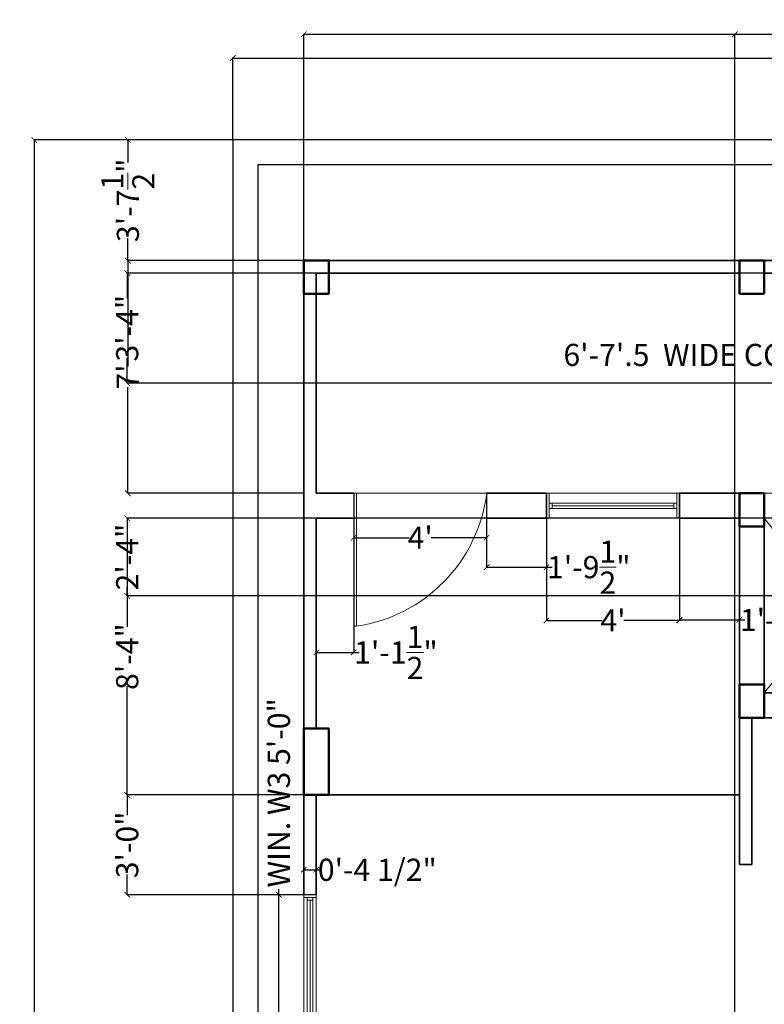
# Model space of a CAD drawing. Units: inches. Extents: x 490 to 1091, y 501 to 1322.
# Tile 4 of 5: x 490 to 759, y 959 to 1314. Entities that reach past the tile are written whole.
import ezdxf

# ---------------------------------------------------------------- set-up
doc = ezdxf.new("R2010")
doc.units = ezdxf.units.IN
doc.header["$MEASUREMENT"] = 0
doc.linetypes.add('ACAD_ISO02W100', pattern=[15, 12, -3])
for name, color, linetype, lineweight in [('A-ANNO-DIMS', 2, 'Continuous', 18), ('A-AREA-IDEN', 7, 'Continuous', 25), ('A-COLS', 12, 'Continuous', 50), ('A-DOOR', 3, 'Continuous', 20), ('A-EQPM-EVTR', 152, 'Continuous', 20), ('A-EQPM-EVTR-HIDN', 152, 'ACAD_ISO02W100', 13), ('A-GLAZ', 4, 'Continuous', 18), ('A-WALL', 7, 'Continuous', 35), ('C-PROP', 8, 'Continuous', 25)]:
    doc.layers.add(name, color=color, linetype=linetype, lineweight=lineweight)
doc.styles.get("Standard").update_dxf_attribs({"font": 'arial.ttf'})
doc.dimstyles.get("Standard").update_dxf_attribs({"dimtxt": 8, "dimasz": 2, "dimexe": 0.18, "dimexo": 0.0625, "dimgap": 0.09, "dimtad": 0, "dimdec": 1, "dimzin": 0, "dimdsep": 46, "dimlunit": 4, "dimtxsty": 'Standard', "dimblk": 'ARCHTICK', "dimcen": 0.09, "dimadec": 0, "dimazin": 0, "dimtfac": 1, "dimtdec": 1, "dimtofl": 0, "dimtmove": 0, "dimatfit": 3, "dimldrblk": 'ARCHTICK', "dimfxl": 1, "dimtolj": 1, "dimtzin": 0, "dimarcsym": 0})

# ---------------------------------------------------------------- blocks, each defined once
blk = doc.blocks.new('_ArchTick')
at = {"color": 0, "linetype": 'ByBlock', "const_width": 0.15}
blk.add_lwpolyline([(-0.5, -0.5), (0.5, 0.5)], dxfattribs=at)
blk = doc.blocks.new('*D2')
at = {"layer": 'A-ANNO-DIMS', "color": 0, "lineweight": -2, "transparency": 16777216}
for p, q in [((592.81, 1227.28), (529.2, 1227.28)), ((529.38, 1227.28), (529.38, 1189.02)), ((529.38, 1143.28), (529.38, 1181.55)), ((592.81, 1143.28), (529.2, 1143.28))]:
    blk.add_line(p, q, dxfattribs=at)
at = {"layer": 'Defpoints', "color": 0, "transparency": 16777216}
for p in [(592.87, 1227.28), (529.38, 1143.28), (592.87, 1143.28)]:
    blk.add_point(p, dxfattribs=at)
at = {"layer": 'A-ANNO-DIMS', "color": 0, "lineweight": -2, "transparency": 16777216, "xscale": 2, "yscale": 2, "zscale": 2}
for p, rotation in [((529.38, 1227.28), 90), ((529.38, 1143.28), 270)]:
    blk.add_blockref('_ArchTick', p, dxfattribs=dict(at, rotation=rotation))
at = {"layer": 'A-ANNO-DIMS', "color": 0, "transparency": 16777216, "insert": (529.38, 1185.28), "char_height": 8, "attachment_point": 5, "rotation": 90}
blk.add_mtext("\\A1;7'", dxfattribs=at)
blk = doc.blocks.new('*D3')
at = {"layer": 'A-ANNO-DIMS', "color": 0, "lineweight": -2, "transparency": 16777216}
for p, q in [((567.27, 1270.95), (567.27, 1300.61)), ((567.27, 1300.43), (800.23, 1300.43)), ((1047.27, 1300.43), (814.31, 1300.43)), ((1047.27, 1270.95), (1047.27, 1300.61))]:
    blk.add_line(p, q, dxfattribs=at)
at = {"layer": 'Defpoints', "color": 0, "transparency": 16777216}
for p in [(567.27, 1300.43), (567.27, 1270.88), (1047.27, 1270.88)]:
    blk.add_point(p, dxfattribs=at)
at = {"layer": 'A-ANNO-DIMS', "color": 0, "lineweight": -2, "transparency": 16777216, "xscale": 2, "yscale": 2, "zscale": 2, "rotation": 180}
blk.add_blockref('_ArchTick', (567.27, 1300.43), dxfattribs=at)
at = {"layer": 'A-ANNO-DIMS', "color": 0, "lineweight": -2, "transparency": 16777216, "xscale": 2, "yscale": 2, "zscale": 2}
blk.add_blockref('_ArchTick', (1047.27, 1300.43), dxfattribs=at)
at = {"layer": 'A-ANNO-DIMS', "color": 0, "transparency": 16777216, "insert": (807.27, 1300.43), "char_height": 8, "attachment_point": 5}
blk.add_mtext("\\A1;40'", dxfattribs=at)
blk = doc.blocks.new('*D4')
at = {"layer": 'A-ANNO-DIMS', "color": 0, "lineweight": -2, "transparency": 16777216}
for p, q in [((567.21, 1270.88), (495.41, 1270.88)), ((495.59, 1270.88), (495.59, 917.79)), ((495.59, 550.88), (495.59, 903.98)), ((567.21, 550.88), (495.41, 550.88))]:
    blk.add_line(p, q, dxfattribs=at)
at = {"layer": 'Defpoints', "color": 0, "transparency": 16777216}
for p in [(567.27, 1270.88), (495.59, 550.88), (567.27, 550.88)]:
    blk.add_point(p, dxfattribs=at)
at = {"layer": 'A-ANNO-DIMS', "color": 0, "lineweight": -2, "transparency": 16777216, "xscale": 2, "yscale": 2, "zscale": 2}
for p, rotation in [((495.59, 1270.88), 90), ((495.59, 550.88), 270)]:
    blk.add_blockref('_ArchTick', p, dxfattribs=dict(at, rotation=rotation))
at = {"layer": 'A-ANNO-DIMS', "color": 0, "transparency": 16777216, "insert": (495.59, 910.88), "char_height": 8, "attachment_point": 5, "rotation": 90}
blk.add_mtext("\\A1;60'", dxfattribs=at)
blk = doc.blocks.new('bnfgfhvhm')
for p, q in [((1106.43, 1203.63), (1115.43, 1203.63)), ((1106.43, 1191.63), (1106.43, 1203.63)), ((1115.43, 1203.63), (1115.43, 1191.63)), ((1115.43, 1191.63), (1106.43, 1191.63))]:
    blk.add_line(p, q)
blk = doc.blocks.new('ghthyjutyut')
for p, q in [((1385.5, 1212.32), (1433.5, 1212.32)), ((1385.5, 1203.32), (1385.5, 1212.32)), ((1386.5, 1203.32), (1386.5, 1212.32)), ((1432.5, 1212.32), (1432.5, 1203.32)), ((1433.5, 1212.32), (1433.5, 1203.32)), ((1386.5, 1208.82), (1432.5, 1208.82)), ((1387.5, 1206.82), (1387.5, 1208.82)), ((1431.5, 1208.82), (1431.5, 1206.82)), ((1386.5, 1206.82), (1432.5, 1206.82)), ((1387.5, 1207.82), (1431.5, 1207.82)), ((1433.5, 1203.32), (1385.5, 1203.32))]:
    blk.add_line(p, q)
blk = doc.blocks.new('jcjg  bmvh')
for p, q in [((1232.66, 1066.6), (1223.66, 1066.6)), ((1223.66, 1066.6), (1223.66, 1042.6)), ((1232.66, 1042.6), (1232.66, 1066.6)), ((1223.66, 1042.6), (1232.66, 1042.6))]:
    blk.add_line(p, q)
blk = doc.blocks.new('ggnhgjgfjhgjjjjjjjj')
for p, q in [((597.37, 998.37), (592.87, 998.37)), ((592.87, 998.37), (592.87, 938.37)), ((597.37, 998.37), (592.87, 998.37)), ((597.37, 997.37), (592.87, 997.37)), ((594.12, 997.37), (594.12, 939.37)), ((596.12, 996.37), (594.12, 996.37)), ((595.12, 996.37), (595.12, 940.37)), ((596.12, 997.37), (596.12, 939.37)), ((597.37, 938.37), (597.37, 998.37)), ((592.87, 939.37), (597.37, 939.37)), ((594.12, 940.37), (596.12, 940.37)), ((597.37, 938.37), (592.87, 938.37)), ((592.87, 938.37), (597.37, 938.37))]:
    blk.add_line(p, q)
blk = doc.blocks.new("door4'")
for p, q in [((1439.4, 1060.56), (1439.4, 1108.56)), ((1439.4, 1108.56), (1440.4, 1108.56)), ((1440.4, 1108.56), (1440.4, 1060.56)), ((1439.4, 1060.56), (1487.4, 1060.56))]:
    blk.add_line(p, q)
blk.add_arc((1432.28, 1053.6), 55.56, 7.2031, 81.5907)
blk = doc.blocks.new('*D26')
at = {"layer": 'A-ANNO-DIMS', "color": 0, "lineweight": -2, "transparency": 16777216}
for p, q in [((728.47, 1134.22), (728.47, 1097.37)), ((750.07, 1134.22), (750.07, 1097.37)), ((728.47, 1097.55), (750.07, 1097.55)), ((750.07, 1097.55), (752.07, 1097.55))]:
    blk.add_line(p, q, dxfattribs=at)
at = {"layer": 'Defpoints', "color": 0, "transparency": 16777216}
for p in [(728.47, 1134.28), (750.07, 1134.28), (750.07, 1097.55)]:
    blk.add_point(p, dxfattribs=at)
at = {"layer": 'A-ANNO-DIMS', "color": 0, "lineweight": -2, "transparency": 16777216, "xscale": 2, "yscale": 2, "zscale": 2, "rotation": 180}
blk.add_blockref('_ArchTick', (728.47, 1097.55), dxfattribs=at)
at = {"layer": 'A-ANNO-DIMS', "color": 0, "lineweight": -2, "transparency": 16777216, "xscale": 2, "yscale": 2, "zscale": 2}
blk.add_blockref('_ArchTick', (750.07, 1097.55), dxfattribs=at)
at = {"layer": 'A-ANNO-DIMS', "color": 0, "transparency": 16777216, "insert": (765.33, 1097.55), "char_height": 8, "attachment_point": 5}
blk.add_mtext('\\A1;1\'-9{\\H1x;\\S1/2;}"', dxfattribs=at)
blk = doc.blocks.new('*D27')
at = {"layer": 'A-ANNO-DIMS', "color": 0, "lineweight": -2, "transparency": 16777216}
for p, q in [((680.47, 1134.22), (680.47, 1097.22)), ((728.47, 1134.22), (728.47, 1097.22)), ((680.47, 1097.4), (700.54, 1097.4)), ((728.47, 1097.4), (708.4, 1097.4))]:
    blk.add_line(p, q, dxfattribs=at)
at = {"layer": 'Defpoints', "color": 0, "transparency": 16777216}
for p in [(680.47, 1134.28), (728.47, 1134.28), (680.47, 1097.4)]:
    blk.add_point(p, dxfattribs=at)
at = {"layer": 'A-ANNO-DIMS', "color": 0, "lineweight": -2, "transparency": 16777216, "xscale": 2, "yscale": 2, "zscale": 2, "rotation": 180}
blk.add_blockref('_ArchTick', (680.47, 1097.4), dxfattribs=at)
at = {"layer": 'A-ANNO-DIMS', "color": 0, "lineweight": -2, "transparency": 16777216, "xscale": 2, "yscale": 2, "zscale": 2}
blk.add_blockref('_ArchTick', (728.47, 1097.4), dxfattribs=at)
at = {"layer": 'A-ANNO-DIMS', "color": 0, "transparency": 16777216, "insert": (704.47, 1097.4), "char_height": 8, "attachment_point": 5}
blk.add_mtext("\\A1;4'", dxfattribs=at)
blk = doc.blocks.new('*D28')
at = {"layer": 'A-ANNO-DIMS', "color": 0, "lineweight": -2, "transparency": 16777216}
for p, q in [((658.87, 1134.22), (658.87, 1116.44)), ((680.47, 1134.22), (680.47, 1116.44)), ((658.87, 1116.62), (680.47, 1116.62)), ((680.47, 1116.62), (682.47, 1116.62))]:
    blk.add_line(p, q, dxfattribs=at)
at = {"layer": 'Defpoints', "color": 0, "transparency": 16777216}
for p in [(658.87, 1134.28), (680.47, 1134.28), (680.47, 1116.62)]:
    blk.add_point(p, dxfattribs=at)
at = {"layer": 'A-ANNO-DIMS', "color": 0, "lineweight": -2, "transparency": 16777216, "xscale": 2, "yscale": 2, "zscale": 2, "rotation": 180}
blk.add_blockref('_ArchTick', (658.87, 1116.62), dxfattribs=at)
at = {"layer": 'A-ANNO-DIMS', "color": 0, "lineweight": -2, "transparency": 16777216, "xscale": 2, "yscale": 2, "zscale": 2}
blk.add_blockref('_ArchTick', (680.47, 1116.62), dxfattribs=at)
at = {"layer": 'A-ANNO-DIMS', "color": 0, "transparency": 16777216, "insert": (695.73, 1116.62), "char_height": 8, "attachment_point": 5}
blk.add_mtext('\\A1;1\'-9{\\H1x;\\S1/2;}"', dxfattribs=at)
blk = doc.blocks.new('*D29')
at = {"layer": 'A-ANNO-DIMS', "color": 0, "lineweight": -2, "transparency": 16777216}
for p, q in [((610.87, 1143.22), (610.87, 1127.07)), ((658.87, 1143.22), (658.87, 1127.07)), ((610.87, 1127.25), (630.94, 1127.25)), ((658.87, 1127.25), (638.8, 1127.25))]:
    blk.add_line(p, q, dxfattribs=at)
at = {"layer": 'Defpoints', "color": 0, "transparency": 16777216}
for p in [(610.87, 1143.28), (658.87, 1143.28), (658.87, 1127.25)]:
    blk.add_point(p, dxfattribs=at)
at = {"layer": 'A-ANNO-DIMS', "color": 0, "lineweight": -2, "transparency": 16777216, "xscale": 2, "yscale": 2, "zscale": 2, "rotation": 180}
blk.add_blockref('_ArchTick', (610.87, 1127.25), dxfattribs=at)
at = {"layer": 'A-ANNO-DIMS', "color": 0, "lineweight": -2, "transparency": 16777216, "xscale": 2, "yscale": 2, "zscale": 2}
blk.add_blockref('_ArchTick', (658.87, 1127.25), dxfattribs=at)
at = {"layer": 'A-ANNO-DIMS', "color": 0, "transparency": 16777216, "insert": (634.87, 1127.25), "char_height": 8, "attachment_point": 5}
blk.add_mtext("\\A1;4'", dxfattribs=at)
blk = doc.blocks.new('*D30')
at = {"layer": 'A-ANNO-DIMS', "color": 0, "lineweight": -2, "transparency": 16777216}
for p, q in [((597.37, 1134.22), (597.37, 1085.65)), ((610.87, 1134.22), (610.87, 1085.65)), ((597.37, 1085.83), (610.87, 1085.83)), ((610.87, 1085.83), (612.87, 1085.83))]:
    blk.add_line(p, q, dxfattribs=at)
at = {"layer": 'Defpoints', "color": 0, "transparency": 16777216}
for p in [(597.37, 1134.28), (610.87, 1134.28), (610.87, 1085.83)]:
    blk.add_point(p, dxfattribs=at)
at = {"layer": 'A-ANNO-DIMS', "color": 0, "lineweight": -2, "transparency": 16777216, "xscale": 2, "yscale": 2, "zscale": 2, "rotation": 180}
blk.add_blockref('_ArchTick', (597.37, 1085.83), dxfattribs=at)
at = {"layer": 'A-ANNO-DIMS', "color": 0, "lineweight": -2, "transparency": 16777216, "xscale": 2, "yscale": 2, "zscale": 2}
blk.add_blockref('_ArchTick', (610.87, 1085.83), dxfattribs=at)
at = {"layer": 'A-ANNO-DIMS', "color": 0, "transparency": 16777216, "insert": (626.13, 1085.83), "char_height": 8, "attachment_point": 5}
blk.add_mtext('\\A1;1\'-1{\\H1x;\\S1/2;}"', dxfattribs=at)
blk = doc.blocks.new('*D35')
at = {"layer": 'A-ANNO-DIMS', "color": 0, "lineweight": -2, "transparency": 16777216}
for p, q in [((567.21, 1270.88), (529.2, 1270.88)), ((529.38, 1270.88), (529.38, 1262.72)), ((529.38, 1227.28), (529.38, 1235.45)), ((567.21, 1227.28), (529.2, 1227.28))]:
    blk.add_line(p, q, dxfattribs=at)
at = {"layer": 'Defpoints', "color": 0, "transparency": 16777216}
for p in [(567.27, 1270.88), (529.38, 1227.28), (567.27, 1227.28)]:
    blk.add_point(p, dxfattribs=at)
at = {"layer": 'A-ANNO-DIMS', "color": 0, "lineweight": -2, "transparency": 16777216, "xscale": 2, "yscale": 2, "zscale": 2}
for p, rotation in [((529.38, 1270.88), 90), ((529.38, 1227.28), 270)]:
    blk.add_blockref('_ArchTick', p, dxfattribs=dict(at, rotation=rotation))
at = {"layer": 'A-ANNO-DIMS', "color": 0, "transparency": 16777216, "insert": (529.38, 1249.08), "char_height": 8, "attachment_point": 5, "rotation": 90}
blk.add_mtext('\\A1;3\'-7{\\H1x;\\S1/2;}"', dxfattribs=at)
blk = doc.blocks.new('*D62')
at = {"layer": 'A-ANNO-DIMS', "color": 0, "lineweight": -2, "transparency": 16777216}
for p, q in [((583.87, 998.37), (583.87, 1000.37)), ((592.81, 998.37), (583.69, 998.37)), ((583.87, 938.37), (583.87, 998.37)), ((592.81, 938.37), (583.69, 938.37))]:
    blk.add_line(p, q, dxfattribs=at)
at = {"layer": 'Defpoints', "color": 0, "transparency": 16777216}
for p in [(583.87, 998.37), (592.87, 998.37), (592.87, 938.37)]:
    blk.add_point(p, dxfattribs=at)
at = {"layer": 'A-ANNO-DIMS', "color": 0, "lineweight": -2, "transparency": 16777216, "xscale": 2, "yscale": 2, "zscale": 2}
for p, rotation in [((583.87, 998.37), 90), ((583.87, 938.37), 270)]:
    blk.add_blockref('_ArchTick', p, dxfattribs=dict(at, rotation=rotation))
at = {"layer": 'A-ANNO-DIMS', "color": 0, "transparency": 16777216, "insert": (583.87, 1035.16), "char_height": 8, "attachment_point": 5, "rotation": 90}
blk.add_mtext('\\A1;WIN. W3 5\'-0"', dxfattribs=at)
blk = doc.blocks.new('*D63')
at = {"layer": 'A-ANNO-DIMS', "color": 0, "lineweight": -2, "transparency": 16777216}
for p, q in [((592.87, 998.43), (592.87, 1007.55)), ((592.87, 1007.37), (597.37, 1007.37)), ((597.37, 998.43), (597.37, 1007.55)), ((597.37, 1007.37), (599.37, 1007.37))]:
    blk.add_line(p, q, dxfattribs=at)
at = {"layer": 'Defpoints', "color": 0, "transparency": 16777216}
for p in [(597.37, 1007.37), (592.87, 998.37), (597.37, 998.37)]:
    blk.add_point(p, dxfattribs=at)
at = {"layer": 'A-ANNO-DIMS', "color": 0, "lineweight": -2, "transparency": 16777216, "xscale": 2, "yscale": 2, "zscale": 2, "rotation": 180}
blk.add_blockref('_ArchTick', (592.87, 1007.37), dxfattribs=at)
at = {"layer": 'A-ANNO-DIMS', "color": 0, "lineweight": -2, "transparency": 16777216, "xscale": 2, "yscale": 2, "zscale": 2}
blk.add_blockref('_ArchTick', (597.37, 1007.37), dxfattribs=at)
at = {"layer": 'A-ANNO-DIMS', "color": 0, "transparency": 16777216, "insert": (619.41, 1007.37), "char_height": 8, "attachment_point": 5}
blk.add_mtext('\\A1;0\'-4 1/2"', dxfattribs=at)
blk = doc.blocks.new('*D64')
at = {"layer": 'A-ANNO-DIMS', "color": 0, "lineweight": -2, "transparency": 16777216}
for p, q in [((592.87, 1227.35), (592.87, 1309.19)), ((592.87, 1309.01), (793.44, 1309.01)), ((1021.67, 1309.01), (821.1, 1309.01)), ((1021.67, 1227.35), (1021.67, 1309.19))]:
    blk.add_line(p, q, dxfattribs=at)
at = {"layer": 'Defpoints', "color": 0, "transparency": 16777216}
for p in [(1021.67, 1309.01), (592.87, 1227.28), (1021.67, 1227.28)]:
    blk.add_point(p, dxfattribs=at)
at = {"layer": 'A-ANNO-DIMS', "color": 0, "lineweight": -2, "transparency": 16777216, "xscale": 2, "yscale": 2, "zscale": 2, "rotation": 180}
blk.add_blockref('_ArchTick', (592.87, 1309.01), dxfattribs=at)
at = {"layer": 'A-ANNO-DIMS', "color": 0, "lineweight": -2, "transparency": 16777216, "xscale": 2, "yscale": 2, "zscale": 2}
blk.add_blockref('_ArchTick', (1021.67, 1309.01), dxfattribs=at)
at = {"layer": 'A-ANNO-DIMS', "color": 0, "transparency": 16777216, "insert": (807.27, 1309.01), "char_height": 8, "attachment_point": 5}
blk.add_mtext('\\A1;35\'-9"', dxfattribs=at)
blk = doc.blocks.new('*D70')
at = {"layer": 'A-ANNO-DIMS', "color": 0, "lineweight": -2, "transparency": 16777216}
for p, q in [((824.61, 1222.78), (528.96, 1222.78)), ((529.14, 1222.78), (529.14, 1213.63)), ((529.14, 1183.03), (529.14, 1192.19)), ((824.61, 1183.03), (528.96, 1183.03))]:
    blk.add_line(p, q, dxfattribs=at)
at = {"layer": 'Defpoints', "color": 0, "transparency": 16777216}
for p in [(824.67, 1222.78), (529.14, 1183.03), (824.67, 1183.03)]:
    blk.add_point(p, dxfattribs=at)
at = {"layer": 'A-ANNO-DIMS', "color": 0, "lineweight": -2, "transparency": 16777216, "xscale": 2, "yscale": 2, "zscale": 2}
for p, rotation in [((529.14, 1222.78), 90), ((529.14, 1183.03), 270)]:
    blk.add_blockref('_ArchTick', p, dxfattribs=dict(at, rotation=rotation))
at = {"layer": 'A-ANNO-DIMS', "color": 0, "transparency": 16777216, "insert": (529.14, 1202.91), "char_height": 8, "attachment_point": 5, "rotation": 90}
blk.add_mtext('\\A1;3\'-4"', dxfattribs=at)
blk = doc.blocks.new('*D72')
at = {"layer": 'A-ANNO-DIMS', "color": 0, "lineweight": -2, "transparency": 16777216}
for p, q in [((823.01, 1134.28), (528.96, 1134.28)), ((529.14, 1134.28), (529.14, 1131.08)), ((529.14, 1106.28), (529.14, 1109.49)), ((823.01, 1106.28), (528.96, 1106.28))]:
    blk.add_line(p, q, dxfattribs=at)
at = {"layer": 'Defpoints', "color": 0, "transparency": 16777216}
for p in [(823.07, 1134.28), (529.14, 1106.28), (823.07, 1106.28)]:
    blk.add_point(p, dxfattribs=at)
at = {"layer": 'A-ANNO-DIMS', "color": 0, "lineweight": -2, "transparency": 16777216, "xscale": 2, "yscale": 2, "zscale": 2}
for p, rotation in [((529.14, 1134.28), 90), ((529.14, 1106.28), 270)]:
    blk.add_blockref('_ArchTick', p, dxfattribs=dict(at, rotation=rotation))
at = {"layer": 'A-ANNO-DIMS', "color": 0, "transparency": 16777216, "insert": (529.14, 1120.28), "char_height": 8, "attachment_point": 5, "rotation": 90}
blk.add_mtext('\\A1;2\'-4"', dxfattribs=at)
blk = doc.blocks.new('*D74')
at = {"layer": 'A-ANNO-DIMS', "color": 0, "lineweight": -2, "transparency": 16777216}
for p, q in [((597.31, 1134.28), (528.96, 1134.28)), ((529.14, 1134.28), (529.14, 1095.06)), ((529.14, 1034.37), (529.14, 1073.6)), ((601.81, 1034.37), (528.96, 1034.37))]:
    blk.add_line(p, q, dxfattribs=at)
at = {"layer": 'Defpoints', "color": 0, "transparency": 16777216}
for p in [(597.37, 1134.28), (529.14, 1034.37), (601.87, 1034.37)]:
    blk.add_point(p, dxfattribs=at)
at = {"layer": 'A-ANNO-DIMS', "color": 0, "lineweight": -2, "transparency": 16777216, "xscale": 2, "yscale": 2, "zscale": 2}
for p, rotation in [((529.14, 1134.28), 90), ((529.14, 1034.37), 270)]:
    blk.add_blockref('_ArchTick', p, dxfattribs=dict(at, rotation=rotation))
at = {"layer": 'A-ANNO-DIMS', "color": 0, "transparency": 16777216, "insert": (529.14, 1084.33), "char_height": 8, "attachment_point": 5, "rotation": 90}
blk.add_mtext('\\A1;8\'-4"', dxfattribs=at)
blk = doc.blocks.new('*D75')
at = {"layer": 'A-ANNO-DIMS', "color": 0, "lineweight": -2, "transparency": 16777216}
for p, q in [((597.31, 1034.37), (528.96, 1034.37)), ((529.14, 1034.37), (529.14, 1027.09)), ((529.14, 998.37), (529.14, 1005.65)), ((597.31, 998.37), (528.96, 998.37))]:
    blk.add_line(p, q, dxfattribs=at)
at = {"layer": 'Defpoints', "color": 0, "transparency": 16777216}
for p in [(529.14, 1034.37), (597.37, 1034.37), (597.37, 998.37)]:
    blk.add_point(p, dxfattribs=at)
at = {"layer": 'A-ANNO-DIMS', "color": 0, "lineweight": -2, "transparency": 16777216, "xscale": 2, "yscale": 2, "zscale": 2}
for p, rotation in [((529.14, 1034.37), 90), ((529.14, 998.37), 270)]:
    blk.add_blockref('_ArchTick', p, dxfattribs=dict(at, rotation=rotation))
at = {"layer": 'A-ANNO-DIMS', "color": 0, "transparency": 16777216, "insert": (529.14, 1016.37), "char_height": 8, "attachment_point": 5, "rotation": 90}
blk.add_mtext('\\A1;3\'-0"', dxfattribs=at)
blk = doc.blocks.new('*D76')
at = {"layer": 'A-ANNO-DIMS', "color": 0, "lineweight": -2, "transparency": 16777216}
for p, q in [((748.47, 802.15), (748.47, 1309.19)), ((748.47, 1309.01), (775.72, 1309.01)), ((830.67, 1309.01), (803.42, 1309.01)), ((830.67, 794.15), (830.67, 1309.19))]:
    blk.add_line(p, q, dxfattribs=at)
at = {"layer": 'Defpoints', "color": 0, "transparency": 16777216}
for p in [(830.67, 1309.01), (748.47, 802.08), (830.67, 794.08)]:
    blk.add_point(p, dxfattribs=at)
at = {"layer": 'A-ANNO-DIMS', "color": 0, "lineweight": -2, "transparency": 16777216, "xscale": 2, "yscale": 2, "zscale": 2, "rotation": 180}
blk.add_blockref('_ArchTick', (748.47, 1309.01), dxfattribs=at)
at = {"layer": 'A-ANNO-DIMS', "color": 0, "lineweight": -2, "transparency": 16777216, "xscale": 2, "yscale": 2, "zscale": 2}
blk.add_blockref('_ArchTick', (830.67, 1309.01), dxfattribs=at)
at = {"layer": 'A-ANNO-DIMS', "color": 0, "transparency": 16777216, "insert": (789.57, 1309.01), "char_height": 8, "attachment_point": 5}
blk.add_mtext('\\A1;6\'-10"', dxfattribs=at)

msp = doc.modelspace()

# ---------------------------------------------------------------- linework, layer by layer
at = {"layer": 'A-DOOR'}
for p, q in [((610.87, 1143.28), (610.87, 1134.28)), ((658.87, 1143.28), (658.87, 1134.28))]:
    msp.add_line(p, q, dxfattribs=at)
at = {"layer": 'A-EQPM-EVTR'}
for p, q in [((759.07, 1143.28), (768.07, 1143.28)), ((768.07, 1134.28), (759.07, 1134.28))]:
    msp.add_line(p, q, dxfattribs=at)
at = {"layer": 'A-EQPM-EVTR-HIDN'}
for p, q in [((759.07, 1134.28), (810.07, 1071.28)), ((810.07, 1134.28), (759.07, 1071.28))]:
    msp.add_line(p, q, dxfattribs=at)
at = {"layer": 'A-WALL'}
for p, q in [((592.87, 1227.28), (592.87, 998.37)), ((1021.67, 1227.28), (592.87, 1227.28)), ((597.37, 1222.78), (597.37, 1143.28)), ((750.07, 1222.78), (597.37, 1222.78)), ((810.07, 1222.78), (759.07, 1222.78)), ((610.87, 1143.28), (597.37, 1143.28)), ((680.47, 1143.28), (658.87, 1143.28)), ((680.47, 1134.28), (680.47, 1143.28)), ((728.47, 1143.28), (728.47, 1134.28)), ((759.07, 1143.28), (728.47, 1143.28)), ((750.07, 1134.28), (750.07, 1143.28)), ((597.37, 1134.28), (610.87, 1134.28)), ((597.37, 1134.28), (597.37, 1058.37)), ((658.87, 1134.28), (680.47, 1134.28)), ((728.47, 1134.28), (750.07, 1134.28)), ((750.07, 1134.28), (750.07, 1062.28)), ((759.07, 1134.28), (759.07, 1071.28)), ((759.07, 1071.28), (810.07, 1071.28)), ((750.07, 1062.28), (819.07, 1062.28)), ((750.07, 1062.28), (750.07, 1009.28)), ((754.57, 1009.28), (754.57, 1062.28)), ((750.07, 1034.37), (592.87, 1034.37)), ((597.37, 1034.37), (597.37, 998.37)), ((750.07, 1009.28), (754.57, 1009.28))]:
    msp.add_line(p, q, dxfattribs=at)
at = {"layer": 'C-PROP'}
for p, q in [((1047.27, 1270.88), (567.27, 1270.88)), ((567.27, 1270.88), (567.27, 550.88)), ((576.27, 1261.88), (576.27, 559.88)), ((1038.27, 1261.88), (576.27, 1261.88))]:
    msp.add_line(p, q, dxfattribs=at)

# ---------------------------------------------------------------- block references
at = {"layer": 'A-COLS'}
for name, p in [('bnfgfhvhm', (-513.56, 23.65)), ('bnfgfhvhm', (-356.36, 23.65)), ('bnfgfhvhm', (-356.36, -60.35)), ('bnfgfhvhm', (-356.36, -129.35)), ('jcjg  bmvh', (-630.79, -8.23))]:
    msp.add_blockref(name, p, dxfattribs=at)
at = {"layer": 'A-DOOR', "xscale": -1, "rotation": 180}
msp.add_blockref("door4'", (-828.53, 2203.85), dxfattribs=at)
at = {"layer": 'A-GLAZ'}
for name, p in [('ghthyjutyut', (-705.03, -69.04)), ('ggnhgjgfjhgjjjjjjjj', (0, 0))]:
    msp.add_blockref(name, p, dxfattribs=at)

# ---------------------------------------------------------------- texts
at = {"layer": 'A-AREA-IDEN', "insert": (678.87, 1197.24), "char_height": 8, "attachment_point": 1}
msp.add_mtext_dynamic_manual_height_columns("\\pxqc;6'-7'.5  WIDE CORRIDOR", width=135.1715, gutter_width=40, heights=[0], dxfattribs=at)

# ---------------------------------------------------------------- dimensions: what is measured, and where the dimension line sits
at = {"layer": 'A-ANNO-DIMS'}
for base, p1, p2, override, picture, middle in [((1021.67, 1309.01), (592.87, 1227.28), (1021.67, 1227.28), {"dimdec": 1, "dimlfac": 1, "dimrnd": 0, "dimzin": 1, "dimdsep": 46, "dimlunit": 4, "dimfrac": 2}, '*D64', (807.27, 1309.01)), ((830.67, 1309.01), (748.47, 802.08), (830.67, 794.08), {"dimdec": 1, "dimlfac": 1, "dimrnd": 0, "dimzin": 1, "dimdsep": 46, "dimlunit": 4, "dimfrac": 2}, '*D76', (789.57, 1309.01)), ((567.27, 1300.43), (1047.27, 1270.88), (567.27, 1270.88), {"dimclrd": 0, "dimclre": 0, "dimclrt": 0}, '*D3', (807.27, 1300.43)), ((658.87, 1127.25), (610.87, 1143.28), (658.87, 1143.28), {"dimclrd": 0, "dimclre": 0, "dimclrt": 0}, '*D29', (634.87, 1127.25)), ((610.87, 1085.83), (597.37, 1134.28), (610.87, 1134.28), {"dimclrd": 0, "dimclre": 0, "dimclrt": 0}, '*D30', (626.13, 1085.83)), ((680.47, 1116.62), (658.87, 1134.28), (680.47, 1134.28), {"dimclrd": 0, "dimclre": 0, "dimclrt": 0}, '*D28', (695.73, 1116.62)), ((680.47, 1097.4), (728.47, 1134.28), (680.47, 1134.28), {"dimclrd": 0, "dimclre": 0, "dimclrt": 0}, '*D27', (704.47, 1097.4)), ((750.07, 1097.55), (728.47, 1134.28), (750.07, 1134.28), {"dimclrd": 0, "dimclre": 0, "dimclrt": 0}, '*D26', (765.33, 1097.55)), ((597.37, 1007.37), (592.87, 998.37), (597.37, 998.37), {"dimdec": 1, "dimlfac": 1, "dimrnd": 0, "dimzin": 1, "dimdsep": 46, "dimlunit": 4, "dimfrac": 2}, '*D63', (619.41, 1007.37))]:
    dim = msp.add_linear_dim(base=base, p1=p1, p2=p2, dimstyle='Standard', override=override, dxfattribs=at)
    dim.commit()
    dim.dimension.update_dxf_attribs({"geometry": picture, "text_midpoint": middle})
for base, p1, p2, override, picture, middle in [((495.59, 550.88), (567.27, 1270.88), (567.27, 550.88), {"dimclrd": 0, "dimclre": 0, "dimclrt": 0}, '*D4', (495.59, 910.88)), ((529.38, 1227.28), (567.27, 1270.88), (567.27, 1227.28), {"dimclrd": 0, "dimclre": 0, "dimclrt": 0}, '*D35', (529.38, 1249.08)), ((529.38, 1143.28), (592.87, 1227.28), (592.87, 1143.28), {"dimclrd": 0, "dimclre": 0, "dimclrt": 0}, '*D2', (529.38, 1185.28)), ((529.139808, 1183.034783), (824.669808, 1222.784783), (824.669808, 1183.034783), {"dimdec": 1, "dimlfac": 1, "dimrnd": 0, "dimzin": 1, "dimdsep": 46, "dimlunit": 4, "dimfrac": 2}, '*D70', (529.139808, 1202.909783)), ((529.14, 1106.28), (823.07, 1134.28), (823.07, 1106.28), {"dimdec": 1, "dimlfac": 1, "dimrnd": 0, "dimzin": 1, "dimdsep": 46, "dimlunit": 4, "dimfrac": 2}, '*D72', (529.14, 1120.28)), ((529.14, 1034.37), (597.37, 1134.28), (601.87, 1034.37), {"dimdec": 1, "dimlfac": 1, "dimrnd": 0, "dimzin": 1, "dimdsep": 46, "dimlunit": 4, "dimfrac": 2}, '*D74', (529.14, 1084.33)), ((529.14, 1034.37), (597.37, 998.37), (597.37, 1034.37), {"dimdec": 1, "dimlfac": 1, "dimrnd": 0, "dimzin": 1, "dimdsep": 46, "dimlunit": 4, "dimfrac": 2}, '*D75', (529.14, 1016.37))]:
    dim = msp.add_linear_dim(base=base, p1=p1, p2=p2, angle=90, dimstyle='Standard', override=override, dxfattribs=at)
    dim.commit()
    dim.dimension.update_dxf_attribs({"geometry": picture, "text_midpoint": middle})
dim = msp.add_linear_dim(base=(583.87, 998.37), p1=(592.87, 938.37), p2=(592.87, 998.37), angle=90, text='WIN. W3 <>', dimstyle='Standard', override={"dimdec": 1, "dimlfac": 1, "dimrnd": 0, "dimzin": 1, "dimdsep": 46, "dimlunit": 4, "dimfrac": 2}, dxfattribs=at)
dim.commit()
dim.dimension.update_dxf_attribs({"geometry": '*D62', "text_midpoint": (583.87, 1035.16)})

doc.saveas('drawing.dxf')
